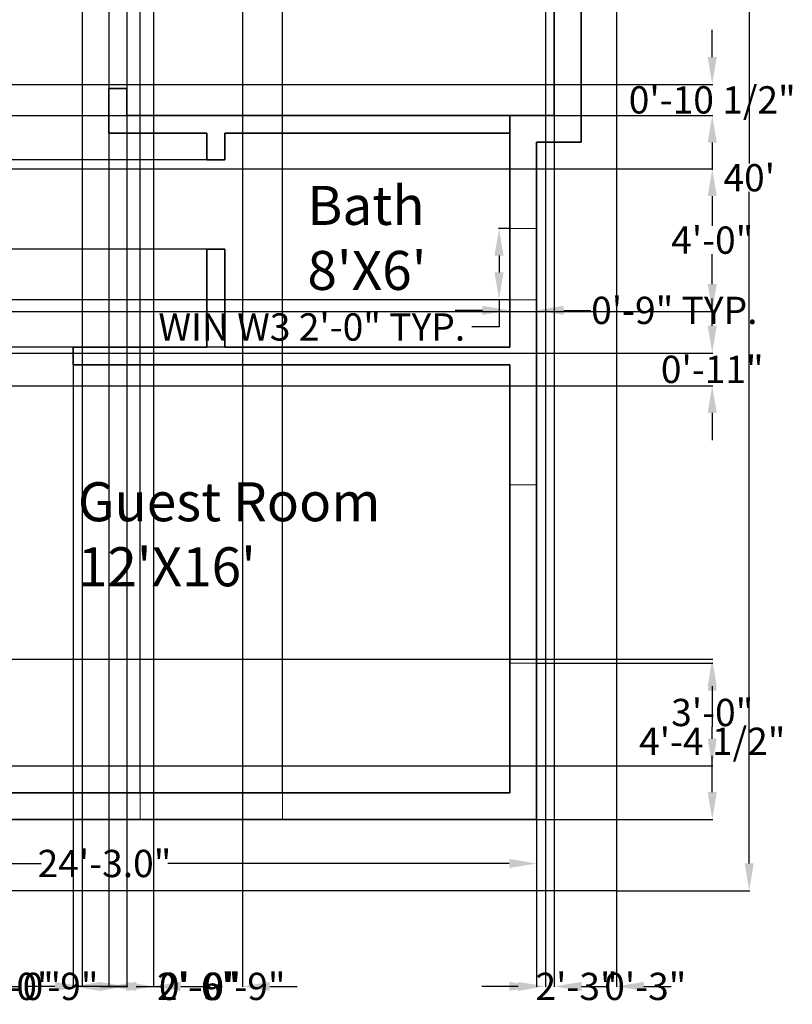
# Model space of a CAD drawing. Units: inches. Extents: x -69 to 558, y -494 to 191.
# Tile 2 of 3: x 289 to 550, y -487 to -155. Entities that reach past the tile are written whole.
import ezdxf

# ---------------------------------------------------------------- set-up
doc = ezdxf.new("R2010")
doc.units = ezdxf.units.IN
doc.header["$MEASUREMENT"] = 0
for name, color, linetype, lineweight in [('A-ANNO-DIMS', 2, 'Continuous', 18), ('A-AREA-IDEN', 7, 'Continuous', 18), ('A-GLAZ', 4, 'Continuous', 18), ('A-WALL', 7, 'Continuous', 35), ('C-PROP', 8, 'Continuous', 25)]:
    doc.layers.add(name, color=color, linetype=linetype, lineweight=lineweight)
doc.styles.get("Standard").update_dxf_attribs({"font": 'arial.ttf'})
doc.dimstyles.get("Standard").update_dxf_attribs({"dimtxt": 9.18, "dimasz": 9.18, "dimexe": 0.18, "dimexo": 0.0625, "dimgap": 0.09, "dimtad": 0, "dimtih": 1, "dimtoh": 1, "dimdec": 1, "dimzin": 0, "dimdsep": 46, "dimlunit": 3, "dimtxsty": 'Standard', "dimcen": 9, "dimadec": 0, "dimazin": 0, "dimtfac": 1, "dimtdec": 1, "dimtofl": 0, "dimtmove": 0, "dimatfit": 3, "dimfxl": 1, "dimtolj": 1, "dimtzin": 0, "dimarcsym": 0})

# ---------------------------------------------------------------- blocks, each defined once
blk = doc.blocks.new('*D8')
at = {"layer": 'A-ANNO-DIMS', "color": 0, "lineweight": -2, "transparency": 16777216}
for p, q in [((490.42, 31.7), (535.2, 31.7)), ((535.02, 22.52), (535.02, -203.53)), ((535.02, -439.12), (535.02, -213.08)), ((490.42, -448.3), (535.2, -448.3))]:
    blk.add_line(p, q, dxfattribs=at)
at = {"layer": 'A-ANNO-DIMS', "color": 0, "transparency": 16777216}
for points in [[(533.49, 22.52), (536.55, 22.52), (535.02, 31.7)], [(533.49, -439.12), (536.55, -439.12), (535.02, -448.3)]]:
    blk.add_solid(points, dxfattribs=at)
at = {"layer": 'Defpoints', "color": 0, "transparency": 16777216}
for p in [(490.36, 31.7), (490.36, -448.3), (535.02, -448.3)]:
    blk.add_point(p, dxfattribs=at)
at = {"layer": 'A-ANNO-DIMS', "color": 0, "transparency": 16777216, "insert": (535.02, -208.3), "char_height": 9.18, "attachment_point": 5}
blk.add_mtext("\\A1;40'", dxfattribs=at)
blk = doc.blocks.new('*D14')
at = {"layer": 'A-ANNO-DIMS', "color": 0, "lineweight": -2, "transparency": 16777216}
for p, q in [((172.36, -424.37), (172.36, -439.31)), ((463.36, -424.37), (463.36, -439.31)), ((181.54, -439.13), (296.57, -439.13)), ((454.18, -439.13), (339.14, -439.13))]:
    blk.add_line(p, q, dxfattribs=at)
at = {"layer": 'A-ANNO-DIMS', "color": 0, "transparency": 16777216}
for points in [[(181.54, -437.6), (181.54, -440.66), (172.36, -439.13)], [(454.18, -437.6), (454.18, -440.66), (463.36, -439.13)]]:
    blk.add_solid(points, dxfattribs=at)
at = {"layer": 'Defpoints', "color": 0, "transparency": 16777216}
for p in [(172.36, -424.3), (463.36, -424.3), (172.36, -439.13)]:
    blk.add_point(p, dxfattribs=at)
at = {"layer": 'A-ANNO-DIMS', "color": 0, "transparency": 16777216, "insert": (317.86, -439.13), "char_height": 9.18, "attachment_point": 5}
blk.add_mtext('\\A1;24\'-3.0"', dxfattribs=at)
blk = doc.blocks.new('WIN-60IN')
blk.add_lwpolyline([(60, 9), (60, 0), (0, 0), (0, 9)], close=True)
blk = doc.blocks.new('WIN-24IN')
blk.add_lwpolyline([(0, 0), (0, 9), (24, 9), (24, 0)], close=True)
blk = doc.blocks.new('*D22')
at = {"layer": 'A-ANNO-DIMS', "color": 0, "lineweight": -2, "transparency": 16777216}
for p, q in [((454.29, -225.35), (450.58, -225.35)), ((450.76, -234.53), (450.76, -240.17)), ((454.29, -249.35), (450.58, -249.35)), ((450.76, -249.35), (450.76, -258.53)), ((450.76, -258.53), (441.58, -258.53))]:
    blk.add_line(p, q, dxfattribs=at)
at = {"layer": 'A-ANNO-DIMS', "color": 0, "transparency": 16777216}
for points in [[(449.23, -234.53), (452.29, -234.53), (450.76, -225.35)], [(449.23, -240.17), (452.29, -240.17), (450.76, -249.35)]]:
    blk.add_solid(points, dxfattribs=at)
at = {"layer": 'Defpoints', "color": 0, "transparency": 16777216}
for p in [(454.36, -225.35), (450.76, -249.35), (454.36, -249.35)]:
    blk.add_point(p, dxfattribs=at)
at = {"layer": 'A-ANNO-DIMS', "color": 0, "transparency": 16777216, "insert": (387.68, -258.53), "char_height": 9.18, "attachment_point": 5}
blk.add_mtext('\\A1;WIN W3 2\'-0" TYP.', dxfattribs=at)
blk = doc.blocks.new('*D23')
at = {"layer": 'A-ANNO-DIMS', "color": 0, "lineweight": -2, "transparency": 16777216}
for p, q in [((454.36, -249.41), (454.36, -253.13)), ((463.36, -249.41), (463.36, -253.13)), ((445.18, -252.95), (436, -252.95)), ((472.54, -252.95), (481.72, -252.95))]:
    blk.add_line(p, q, dxfattribs=at)
at = {"layer": 'A-ANNO-DIMS', "color": 0, "transparency": 16777216}
for points in [[(445.18, -251.42), (445.18, -254.48), (454.36, -252.95)], [(472.54, -251.42), (472.54, -254.48), (463.36, -252.95)]]:
    blk.add_solid(points, dxfattribs=at)
at = {"layer": 'Defpoints', "color": 0, "transparency": 16777216}
for p in [(454.36, -249.35), (463.36, -249.35), (463.36, -252.95)]:
    blk.add_point(p, dxfattribs=at)
at = {"layer": 'A-ANNO-DIMS', "color": 0, "transparency": 16777216, "insert": (509.79, -252.95), "char_height": 9.18, "attachment_point": 5}
blk.add_mtext('\\A1;0\'-9" TYP.', dxfattribs=at)
blk = doc.blocks.new('*D31')
at = {"layer": 'A-ANNO-DIMS', "color": 0, "lineweight": -2, "transparency": 16777216}
for p, q in [((522.557437, -258.12485), (522.557437, -248.94485)), ((158.419937, -267.30485), (522.737437, -267.30485)), ((158.419937, -278.30485), (522.737437, -278.30485)), ((522.557437, -287.48485), (522.557437, -296.66485))]:
    blk.add_line(p, q, dxfattribs=at)
at = {"layer": 'A-ANNO-DIMS', "color": 0, "transparency": 16777216}
for points in [[(521.027437, -258.12485), (524.087437, -258.12485), (522.557437, -267.30485)], [(521.027437, -287.48485), (524.087437, -287.48485), (522.557437, -278.30485)]]:
    blk.add_solid(points, dxfattribs=at)
at = {"layer": 'Defpoints', "color": 0, "transparency": 16777216}
for p in [(158.357437, -267.30485), (158.357437, -278.30485), (522.557437, -278.30485)]:
    blk.add_point(p, dxfattribs=at)
at = {"layer": 'A-ANNO-DIMS', "color": 0, "transparency": 16777216, "insert": (522.557437, -272.80485), "char_height": 9.18, "attachment_point": 5}
blk.add_mtext('\\A1;0\'-11"', dxfattribs=at)
blk = doc.blocks.new('*D33')
at = {"layer": 'A-ANNO-DIMS', "color": 0, "lineweight": -2, "transparency": 16777216}
for p, q in [((329.86, -415.24), (329.86, 64.08)), ((339.04, 63.9), (341.38, 63.9)), ((368.68, 63.9), (366.33, 63.9)), ((377.86, -415.24), (377.86, 64.08))]:
    blk.add_line(p, q, dxfattribs=at)
at = {"layer": 'A-ANNO-DIMS', "color": 0, "transparency": 16777216}
for points in [[(339.04, 65.43), (339.04, 62.37), (329.86, 63.9)], [(368.68, 65.43), (368.68, 62.37), (377.86, 63.9)]]:
    blk.add_solid(points, dxfattribs=at)
at = {"layer": 'Defpoints', "color": 0, "transparency": 16777216}
for p in [(377.86, 63.9), (329.86, -415.3), (377.86, -415.3)]:
    blk.add_point(p, dxfattribs=at)
at = {"layer": 'A-ANNO-DIMS', "color": 0, "transparency": 16777216, "insert": (353.86, 63.9), "char_height": 9.18, "attachment_point": 5}
blk.add_mtext('\\A1;4\'-0"', dxfattribs=at)
blk = doc.blocks.new('*D35')
at = {"layer": 'A-ANNO-DIMS', "color": 0, "lineweight": -2, "transparency": 16777216}
for p, q in [((334.357437, -67.36735), (334.357437, -480.68485)), ((364.357437, -67.36735), (364.357437, -480.68485)), ((325.177437, -480.50485), (315.997437, -480.50485)), ((373.537437, -480.50485), (382.717437, -480.50485))]:
    blk.add_line(p, q, dxfattribs=at)
at = {"layer": 'A-ANNO-DIMS', "color": 0, "transparency": 16777216}
for points in [[(325.177437, -478.97485), (325.177437, -482.03485), (334.357437, -480.50485)], [(373.537437, -478.97485), (373.537437, -482.03485), (364.357437, -480.50485)]]:
    blk.add_solid(points, dxfattribs=at)
at = {"layer": 'Defpoints', "color": 0, "transparency": 16777216}
for p in [(334.357437, -67.30485), (364.357437, -67.30485), (364.357437, -480.50485)]:
    blk.add_point(p, dxfattribs=at)
at = {"layer": 'A-ANNO-DIMS', "color": 0, "transparency": 16777216, "insert": (349.357437, -480.50485), "char_height": 9.18, "attachment_point": 5}
blk.add_mtext('\\A1;2\'-6"', dxfattribs=at)
blk = doc.blocks.new('*D38')
at = {"layer": 'A-ANNO-DIMS', "color": 0, "lineweight": -2, "transparency": 16777216}
for p, q in [((-33.84, -240.17), (-33.84, -230.99)), ((454.29, -249.35), (-34.02, -249.35)), ((454.29, -265.3), (-34.02, -265.3)), ((-33.84, -274.48), (-33.84, -283.66))]:
    blk.add_line(p, q, dxfattribs=at)
at = {"layer": 'A-ANNO-DIMS', "color": 0, "transparency": 16777216}
for points in [[(-35.37, -240.17), (-32.31, -240.17), (-33.84, -249.35)], [(-35.37, -274.48), (-32.31, -274.48), (-33.84, -265.3)]]:
    blk.add_solid(points, dxfattribs=at)
at = {"layer": 'Defpoints', "color": 0, "transparency": 16777216}
for p in [(-33.84, -249.35), (454.36, -249.35), (454.36, -265.3)]:
    blk.add_point(p, dxfattribs=at)
at = {"layer": 'A-ANNO-DIMS', "color": 0, "transparency": 16777216, "insert": (-33.84, -257.33), "char_height": 9.18, "attachment_point": 5}
blk.add_mtext('\\A1;1\'-4"', dxfattribs=at)
blk = doc.blocks.new('*D43')
at = {"layer": 'A-ANNO-DIMS', "color": 0, "lineweight": -2, "transparency": 16777216}
for p, q in [((466.36, -48.37), (466.36, -480.68)), ((469.36, -48.37), (469.36, -480.68)), ((457.18, -480.5), (448, -480.5)), ((478.54, -480.5), (487.72, -480.5))]:
    blk.add_line(p, q, dxfattribs=at)
at = {"layer": 'A-ANNO-DIMS', "color": 0, "transparency": 16777216}
for points in [[(457.18, -478.97), (457.18, -482.03), (466.36, -480.5)], [(478.54, -478.97), (478.54, -482.03), (469.36, -480.5)]]:
    blk.add_solid(points, dxfattribs=at)
at = {"layer": 'Defpoints', "color": 0, "transparency": 16777216}
for p in [(466.36, -48.3), (469.36, -48.3), (469.36, -480.5)]:
    blk.add_point(p, dxfattribs=at)
at = {"layer": 'A-ANNO-DIMS', "color": 0, "transparency": 16777216, "insert": (500.01, -480.5), "char_height": 9.18, "attachment_point": 5}
blk.add_mtext('\\A1;0\'-3"', dxfattribs=at)
blk = doc.blocks.new('*D44')
at = {"layer": 'A-ANNO-DIMS', "color": 0, "lineweight": -2, "transparency": 16777216}
for p, q in [((522.557437, -167.693456), (522.557437, -158.513456)), ((25.419937, -176.873456), (522.737437, -176.873456)), ((25.419937, -187.30485), (522.737437, -187.30485)), ((522.557437, -196.48485), (522.557437, -205.66485))]:
    blk.add_line(p, q, dxfattribs=at)
at = {"layer": 'A-ANNO-DIMS', "color": 0, "transparency": 16777216}
for points in [[(521.027437, -167.693456), (524.087437, -167.693456), (522.557437, -176.873456)], [(521.027437, -196.48485), (524.087437, -196.48485), (522.557437, -187.30485)]]:
    blk.add_solid(points, dxfattribs=at)
at = {"layer": 'Defpoints', "color": 0, "transparency": 16777216}
for p in [(25.357437, -176.873456), (522.557437, -176.873456), (25.357437, -187.30485)]:
    blk.add_point(p, dxfattribs=at)
at = {"layer": 'A-ANNO-DIMS', "color": 0, "transparency": 16777216, "insert": (522.557437, -182.089153), "char_height": 9.18, "attachment_point": 5}
blk.add_mtext('\\A1;0\'-10 1/2"', dxfattribs=at)
blk = doc.blocks.new('*D46')
at = {"layer": 'A-ANNO-DIMS', "color": 0, "lineweight": -2, "transparency": 16777216}
for p, q in [((463.42, -371.72), (522.74, -371.72)), ((522.56, -380.9), (522.56, -393.17)), ((522.56, -415.12), (522.56, -402.85)), ((463.42, -424.3), (522.74, -424.3))]:
    blk.add_line(p, q, dxfattribs=at)
at = {"layer": 'A-ANNO-DIMS', "color": 0, "transparency": 16777216}
for points in [[(521.03, -380.9), (524.09, -380.9), (522.56, -371.72)], [(521.03, -415.12), (524.09, -415.12), (522.56, -424.3)]]:
    blk.add_solid(points, dxfattribs=at)
at = {"layer": 'Defpoints', "color": 0, "transparency": 16777216}
for p in [(463.36, -371.72), (522.56, -371.72), (463.36, -424.3)]:
    blk.add_point(p, dxfattribs=at)
at = {"layer": 'A-ANNO-DIMS', "color": 0, "transparency": 16777216, "insert": (522.56, -398.01), "char_height": 9.18, "attachment_point": 5}
blk.add_mtext('\\A1;4\'-4 1/2"', dxfattribs=at)
blk = doc.blocks.new('*D47')
at = {"layer": 'A-ANNO-DIMS', "color": 0, "lineweight": -2, "transparency": 16777216}
for p, q in [((262.36, -415.24), (262.36, 64.08)), ((271.54, 63.9), (273.12, 63.9)), ((320.68, 63.9), (319.09, 63.9)), ((329.86, -415.24), (329.86, 64.08))]:
    blk.add_line(p, q, dxfattribs=at)
at = {"layer": 'A-ANNO-DIMS', "color": 0, "transparency": 16777216}
for points in [[(271.54, 65.43), (271.54, 62.37), (262.36, 63.9)], [(320.68, 65.43), (320.68, 62.37), (329.86, 63.9)]]:
    blk.add_solid(points, dxfattribs=at)
at = {"layer": 'Defpoints', "color": 0, "transparency": 16777216}
for p in [(329.86, 63.9), (262.36, -415.3), (329.86, -415.3)]:
    blk.add_point(p, dxfattribs=at)
at = {"layer": 'A-ANNO-DIMS', "color": 0, "transparency": 16777216, "insert": (296.11, 63.9), "char_height": 9.18, "attachment_point": 5}
blk.add_mtext('\\A1;5\'-7 1/2"', dxfattribs=at)
blk = doc.blocks.new('*D48')
at = {"layer": 'A-ANNO-DIMS', "color": 0, "lineweight": -2, "transparency": 16777216}
for p, q in [((310.36, -127.37), (310.36, -480.68)), ((319.36, -127.37), (319.36, -480.68)), ((301.18, -480.5), (292, -480.5)), ((328.54, -480.5), (337.72, -480.5))]:
    blk.add_line(p, q, dxfattribs=at)
at = {"layer": 'A-ANNO-DIMS', "color": 0, "transparency": 16777216}
for points in [[(301.18, -478.97), (301.18, -482.03), (310.36, -480.5)], [(328.54, -478.97), (328.54, -482.03), (319.36, -480.5)]]:
    blk.add_solid(points, dxfattribs=at)
at = {"layer": 'Defpoints', "color": 0, "transparency": 16777216}
for p in [(310.36, -127.3), (319.36, -127.3), (319.36, -480.5)]:
    blk.add_point(p, dxfattribs=at)
at = {"layer": 'A-ANNO-DIMS', "color": 0, "transparency": 16777216, "insert": (350.01, -480.5), "char_height": 9.18, "attachment_point": 5}
blk.add_mtext('\\A1;0\'-9"', dxfattribs=at)
blk = doc.blocks.new('*D49')
at = {"layer": 'A-ANNO-DIMS', "color": 0, "lineweight": -2, "transparency": 16777216}
for p, q in [((325.36, -61.37), (325.36, -480.68)), ((334.36, -61.37), (334.36, -480.68)), ((316.18, -480.5), (307, -480.5)), ((343.54, -480.5), (352.72, -480.5))]:
    blk.add_line(p, q, dxfattribs=at)
at = {"layer": 'A-ANNO-DIMS', "color": 0, "transparency": 16777216}
for points in [[(316.18, -478.97), (316.18, -482.03), (325.36, -480.5)], [(343.54, -478.97), (343.54, -482.03), (334.36, -480.5)]]:
    blk.add_solid(points, dxfattribs=at)
at = {"layer": 'Defpoints', "color": 0, "transparency": 16777216}
for p in [(325.36, -61.3), (334.36, -61.3), (334.36, -480.5)]:
    blk.add_point(p, dxfattribs=at)
at = {"layer": 'A-ANNO-DIMS', "color": 0, "transparency": 16777216, "insert": (365.01, -480.5), "char_height": 9.18, "attachment_point": 5}
blk.add_mtext('\\A1;0\'-9"', dxfattribs=at)
blk = doc.blocks.new('*D52')
at = {"layer": 'A-ANNO-DIMS', "color": 0, "lineweight": -2, "transparency": 16777216}
for p, q in [((271.357437, -271.36735), (271.357437, -480.68485)), ((307.357437, -271.36735), (307.357437, -480.68485)), ((262.177437, -480.50485), (252.997437, -480.50485)), ((316.537437, -480.50485), (325.717437, -480.50485))]:
    blk.add_line(p, q, dxfattribs=at)
at = {"layer": 'A-ANNO-DIMS', "color": 0, "transparency": 16777216}
for points in [[(262.177437, -478.97485), (262.177437, -482.03485), (271.357437, -480.50485)], [(316.537437, -478.97485), (316.537437, -482.03485), (307.357437, -480.50485)]]:
    blk.add_solid(points, dxfattribs=at)
at = {"layer": 'Defpoints', "color": 0, "transparency": 16777216}
for p in [(271.357437, -271.30485), (307.357437, -271.30485), (307.357437, -480.50485)]:
    blk.add_point(p, dxfattribs=at)
at = {"layer": 'A-ANNO-DIMS', "color": 0, "transparency": 16777216, "insert": (289.357437, -480.50485), "char_height": 9.18, "attachment_point": 5}
blk.add_mtext('\\A1;3\'-0"', dxfattribs=at)
blk = doc.blocks.new('*D53')
at = {"layer": 'A-ANNO-DIMS', "color": 0, "lineweight": -2, "transparency": 16777216}
for p, q in [((262.36, -271.37), (262.36, -480.68)), ((271.36, -271.37), (271.36, -480.68)), ((253.18, -480.5), (244, -480.5)), ((280.54, -480.5), (289.72, -480.5))]:
    blk.add_line(p, q, dxfattribs=at)
at = {"layer": 'A-ANNO-DIMS', "color": 0, "transparency": 16777216}
for points in [[(253.18, -478.97), (253.18, -482.03), (262.36, -480.5)], [(280.54, -478.97), (280.54, -482.03), (271.36, -480.5)]]:
    blk.add_solid(points, dxfattribs=at)
at = {"layer": 'Defpoints', "color": 0, "transparency": 16777216}
for p in [(262.36, -271.3), (271.36, -271.3), (271.36, -480.5)]:
    blk.add_point(p, dxfattribs=at)
at = {"layer": 'A-ANNO-DIMS', "color": 0, "transparency": 16777216, "insert": (302.01, -480.5), "char_height": 9.18, "attachment_point": 5}
blk.add_mtext('\\A1;0\'-9"', dxfattribs=at)
blk = doc.blocks.new('*D54')
at = {"layer": 'A-ANNO-DIMS', "color": 0, "lineweight": -2, "transparency": 16777216}
for p, q in [((358.29, -202.3), (-34.02, -202.3)), ((-33.84, -211.48), (-33.84, -212.53)), ((-33.84, -223.12), (-33.84, -222.08)), ((358.29, -232.3), (-34.02, -232.3))]:
    blk.add_line(p, q, dxfattribs=at)
at = {"layer": 'A-ANNO-DIMS', "color": 0, "transparency": 16777216}
for points in [[(-35.37, -211.48), (-32.31, -211.48), (-33.84, -202.3)], [(-35.37, -223.12), (-32.31, -223.12), (-33.84, -232.3)]]:
    blk.add_solid(points, dxfattribs=at)
at = {"layer": 'Defpoints', "color": 0, "transparency": 16777216}
for p in [(358.36, -202.3), (-33.84, -232.3), (358.36, -232.3)]:
    blk.add_point(p, dxfattribs=at)
at = {"layer": 'A-ANNO-DIMS', "color": 0, "transparency": 16777216, "insert": (-33.84, -217.3), "char_height": 9.18, "attachment_point": 5}
blk.add_mtext('\\A1;2\'-6"', dxfattribs=at)
blk = doc.blocks.new('*D55')
at = {"layer": 'A-ANNO-DIMS', "color": 0, "lineweight": -2, "transparency": 16777216}
for p, q in [((262.42, -370.3), (522.74, -370.3)), ((522.56, -379.48), (522.56, -383.52)), ((522.56, -397.12), (522.56, -393.09)), ((262.42, -406.3), (522.74, -406.3))]:
    blk.add_line(p, q, dxfattribs=at)
at = {"layer": 'A-ANNO-DIMS', "color": 0, "transparency": 16777216}
for points in [[(521.03, -379.48), (524.09, -379.48), (522.56, -370.3)], [(521.03, -397.12), (524.09, -397.12), (522.56, -406.3)]]:
    blk.add_solid(points, dxfattribs=at)
at = {"layer": 'Defpoints', "color": 0, "transparency": 16777216}
for p in [(262.36, -370.3), (262.36, -406.3), (522.56, -406.3)]:
    blk.add_point(p, dxfattribs=at)
at = {"layer": 'A-ANNO-DIMS', "color": 0, "transparency": 16777216, "insert": (522.56, -388.3), "char_height": 9.18, "attachment_point": 5}
blk.add_mtext('\\A1;3\'-0"', dxfattribs=at)
blk = doc.blocks.new('*D59')
at = {"layer": 'A-ANNO-DIMS', "color": 0, "lineweight": -2, "transparency": 16777216}
for p, q in [((463.357437, -424.36735), (463.357437, -480.68485)), ((490.357437, -448.36735), (490.357437, -480.68485)), ((454.177437, -480.50485), (444.997437, -480.50485)), ((499.537437, -480.50485), (508.717437, -480.50485))]:
    blk.add_line(p, q, dxfattribs=at)
at = {"layer": 'A-ANNO-DIMS', "color": 0, "transparency": 16777216}
for points in [[(454.177437, -478.97485), (454.177437, -482.03485), (463.357437, -480.50485)], [(499.537437, -478.97485), (499.537437, -482.03485), (490.357437, -480.50485)]]:
    blk.add_solid(points, dxfattribs=at)
at = {"layer": 'Defpoints', "color": 0, "transparency": 16777216}
for p in [(463.357437, -424.30485), (490.357437, -448.30485), (490.357437, -480.50485)]:
    blk.add_point(p, dxfattribs=at)
at = {"layer": 'A-ANNO-DIMS', "color": 0, "transparency": 16777216, "insert": (476.857437, -480.50485), "char_height": 9.18, "attachment_point": 5}
blk.add_mtext('\\A1;2\'-3"', dxfattribs=at)
blk = doc.blocks.new('*D60')
at = {"layer": 'A-ANNO-DIMS', "color": 0, "lineweight": -2, "transparency": 16777216}
for p, q in [((122.42, -205.3), (522.74, -205.3)), ((522.56, -214.48), (522.56, -224.53)), ((522.56, -244.12), (522.56, -234.08)), ((122.42, -253.3), (522.74, -253.3))]:
    blk.add_line(p, q, dxfattribs=at)
at = {"layer": 'A-ANNO-DIMS', "color": 0, "transparency": 16777216}
for points in [[(521.03, -214.48), (524.09, -214.48), (522.56, -205.3)], [(521.03, -244.12), (524.09, -244.12), (522.56, -253.3)]]:
    blk.add_solid(points, dxfattribs=at)
at = {"layer": 'Defpoints', "color": 0, "transparency": 16777216}
for p in [(122.36, -205.3), (122.36, -253.3), (522.56, -253.3)]:
    blk.add_point(p, dxfattribs=at)
at = {"layer": 'A-ANNO-DIMS', "color": 0, "transparency": 16777216, "insert": (522.56, -229.3), "char_height": 9.18, "attachment_point": 5}
blk.add_mtext('\\A1;4\'-0"', dxfattribs=at)

msp = doc.modelspace()

# ---------------------------------------------------------------- linework, layer by layer
at = {"layer": 'A-GLAZ'}
msp.add_lwpolyline([(329.86, -424.3), (329.86, -415.3), (377.86, -415.3), (377.86, -424.3)], close=True, dxfattribs=at)
at = {"layer": 'A-WALL'}
for p, q in [((478.36, -196.3), (478.36, -39.3)), ((469.36, -187.3), (469.36, -48.3)), ((319.36, -193.3), (319.36, -178.3)), ((319.36, -178.3), (325.36, -178.3)), ((325.36, -187.3), (325.36, -178.3)), ((325.36, -187.3), (469.36, -187.3)), ((454.36, -265.3), (454.36, -187.3)), ((319.36, -193.3), (352.36, -193.3)), ((352.36, -202.3), (352.36, -193.3)), ((358.36, -202.3), (358.36, -193.3)), ((358.36, -193.3), (454.36, -193.3)), ((463.36, -424.3), (463.36, -196.3)), ((463.36, -196.3), (478.36, -196.3)), ((352.36, -202.3), (358.36, -202.3)), ((352.36, -265.3), (352.36, -232.3)), ((352.36, -232.3), (358.36, -232.3)), ((358.36, -265.3), (358.36, -232.3)), ((307.36, -265.3), (319.36, -265.3)), ((307.36, -271.3), (307.36, -265.3)), ((307.36, -265.3), (352.36, -265.3)), ((358.36, -265.3), (454.36, -265.3)), ((373.36, -265.3), (454.36, -265.3)), ((307.36, -271.3), (454.36, -271.3)), ((454.36, -415.3), (454.36, -271.3)), ((454.36, -415.3), (262.36, -415.3)), ((463.36, -424.3), (172.36, -424.3))]:
    msp.add_line(p, q, dxfattribs=at)
at = {"layer": 'C-PROP'}
for p, q in [((490.36, 31.7), (490.36, -448.3)), ((490.36, -448.3), (-1.64, -448.3))]:
    msp.add_line(p, q, dxfattribs=at)

# ---------------------------------------------------------------- block references
at = {"layer": 'A-GLAZ'}
for name, p, rotation in [('WIN-24IN', (454.36, -225.35), 269.9999999999998), ('WIN-60IN', (463.36, -371.72), 89.99999999999987)]:
    msp.add_blockref(name, p, dxfattribs=dict(at, rotation=rotation))

# ---------------------------------------------------------------- texts
at = {"layer": 'A-AREA-IDEN', "char_height": 13.129, "attachment_point": 1}
for s, insert in [("Bath\\P8'X6'", (386.21, -211.05)), ("Guest Room\\P12'X16'", (308.88, -310.8))]:
    msp.add_mtext_dynamic_manual_height_columns(s, width=125.4475, gutter_width=65.65, heights=[60.44], dxfattribs=dict(at, insert=insert))

# ---------------------------------------------------------------- dimensions: what is measured, and where the dimension line sits
at = {"layer": 'A-ANNO-DIMS'}
for base, p1, p2, override, picture, middle in [((329.86, 63.9), (262.36, -415.3), (329.86, -415.3), {"dimdec": 1, "dimlfac": 1, "dimrnd": 0, "dimzin": 1, "dimdsep": 46, "dimlunit": 4, "dimfrac": 2}, '*D47', (296.11, 63.9)), ((377.86, 63.9), (329.86, -415.3), (377.86, -415.3), {"dimdec": 1, "dimlfac": 1, "dimrnd": 0, "dimzin": 1, "dimdsep": 46, "dimlunit": 4, "dimfrac": 2}, '*D33', (353.86, 63.9)), ((469.36, -480.5), (466.36, -48.3), (469.36, -48.3), {"dimdec": 1, "dimlfac": 1, "dimrnd": 0, "dimzin": 1, "dimdsep": 46, "dimlunit": 4, "dimfrac": 2}, '*D43', (500.01, -480.5)), ((334.36, -480.5), (325.36, -61.3), (334.36, -61.3), {"dimdec": 1, "dimlfac": 1, "dimrnd": 0, "dimzin": 1, "dimdsep": 46, "dimlunit": 4, "dimfrac": 2}, '*D49', (365.01, -480.5)), ((364.36, -480.5), (334.36, -67.3), (364.36, -67.3), {"dimdec": 1, "dimlfac": 1, "dimrnd": 0, "dimzin": 1, "dimdsep": 46, "dimlunit": 4, "dimfrac": 2}, '*D35', (349.36, -480.5)), ((319.36, -480.5), (310.36, -127.3), (319.36, -127.3), {"dimdec": 1, "dimlfac": 1, "dimrnd": 0, "dimzin": 1, "dimdsep": 46, "dimlunit": 4, "dimfrac": 2}, '*D48', (350.01, -480.5)), ((271.36, -480.5), (262.36, -271.3), (271.36, -271.3), {"dimdec": 1, "dimlfac": 1, "dimrnd": 0, "dimzin": 1, "dimdsep": 46, "dimlunit": 4, "dimfrac": 2}, '*D53', (302.01, -480.5)), ((307.36, -480.5), (271.36, -271.3), (307.36, -271.3), {"dimdec": 1, "dimlfac": 1, "dimrnd": 0, "dimzin": 1, "dimdsep": 46, "dimlunit": 4, "dimfrac": 2}, '*D52', (289.36, -480.5)), ((172.36, -439.13), (463.36, -424.3), (172.36, -424.3), {"dimclrd": 0, "dimclre": 0, "dimclrt": 0}, '*D14', (317.86, -439.13)), ((490.36, -480.5), (463.36, -424.3), (490.36, -448.3), {"dimdec": 1, "dimlfac": 1, "dimrnd": 0, "dimzin": 1, "dimdsep": 46, "dimlunit": 4, "dimfrac": 2}, '*D59', (476.86, -480.5))]:
    dim = msp.add_linear_dim(base=base, p1=p1, p2=p2, dimstyle='Standard', override=override, dxfattribs=at)
    dim.commit()
    dim.dimension.update_dxf_attribs({"geometry": picture, "text_midpoint": middle})
for base, p1, p2, override, picture, middle in [((535.02, -448.3), (490.36, 31.7), (490.36, -448.3), {"dimclrd": 0, "dimclre": 0, "dimclrt": 0}, '*D8', (535.02, -208.3)), ((522.56, -176.87), (25.36, -187.3), (25.36, -176.87), {"dimdec": 1, "dimlfac": 1, "dimrnd": 0, "dimzin": 1, "dimdsep": 46, "dimlunit": 4, "dimfrac": 2}, '*D44', (522.56, -182.09)), ((-33.84, -232.3), (358.36, -202.3), (358.36, -232.3), {"dimdec": 1, "dimlfac": 1, "dimrnd": 0, "dimzin": 1, "dimdsep": 46, "dimlunit": 4, "dimfrac": 2}, '*D54', (-33.84, -217.3)), ((522.56, -253.3), (122.36, -205.3), (122.36, -253.3), {"dimdec": 1, "dimlfac": 1, "dimrnd": 0, "dimzin": 1, "dimdsep": 46, "dimlunit": 4, "dimfrac": 2}, '*D60', (522.56, -229.3)), ((-33.8426, -249.3471), (454.3574, -265.3048), (454.3574, -249.3471), {"dimdec": 1, "dimlfac": 1, "dimrnd": 0, "dimzin": 1, "dimdsep": 46, "dimlunit": 4, "dimfrac": 2}, '*D38', (-33.8426, -257.326)), ((522.56, -278.3), (158.36, -267.3), (158.36, -278.3), {"dimdec": 1, "dimlfac": 1, "dimrnd": 0, "dimzin": 1, "dimdsep": 46, "dimlunit": 4, "dimfrac": 2}, '*D31', (522.56, -272.8)), ((522.56, -406.3), (262.36, -370.3), (262.36, -406.3), {"dimdec": 1, "dimlfac": 1, "dimrnd": 0, "dimzin": 1, "dimdsep": 46, "dimlunit": 4, "dimfrac": 2}, '*D55', (522.56, -388.3)), ((522.56, -371.72), (463.36, -424.3), (463.36, -371.72), {"dimdec": 1, "dimlfac": 1, "dimrnd": 0, "dimzin": 1, "dimdsep": 46, "dimlunit": 4, "dimfrac": 2}, '*D46', (522.56, -398.01))]:
    dim = msp.add_linear_dim(base=base, p1=p1, p2=p2, angle=90, dimstyle='Standard', override=override, dxfattribs=at)
    dim.commit()
    dim.dimension.update_dxf_attribs({"geometry": picture, "text_midpoint": middle})
dim = msp.add_linear_dim(base=(450.76, -249.35), p1=(454.36, -225.35), p2=(454.36, -249.35), angle=270, text='WIN W3 <> TYP.', dimstyle='Standard', override={"dimdec": 1, "dimlfac": 1, "dimrnd": 0, "dimzin": 1, "dimdsep": 46, "dimlunit": 4, "dimfrac": 2}, dxfattribs=at)
dim.commit()
dim.dimension.update_dxf_attribs({"geometry": '*D22', "text_midpoint": (387.68, -258.53)})
dim = msp.add_linear_dim(base=(463.36, -252.95), p1=(454.36, -249.35), p2=(463.36, -249.35), text='<> TYP.', dimstyle='Standard', override={"dimdec": 1, "dimlfac": 1, "dimrnd": 0, "dimzin": 1, "dimdsep": 46, "dimlunit": 4, "dimfrac": 2}, dxfattribs=at)
dim.commit()
dim.dimension.update_dxf_attribs({"geometry": '*D23', "text_midpoint": (509.79, -252.95)})

doc.saveas('drawing.dxf')
